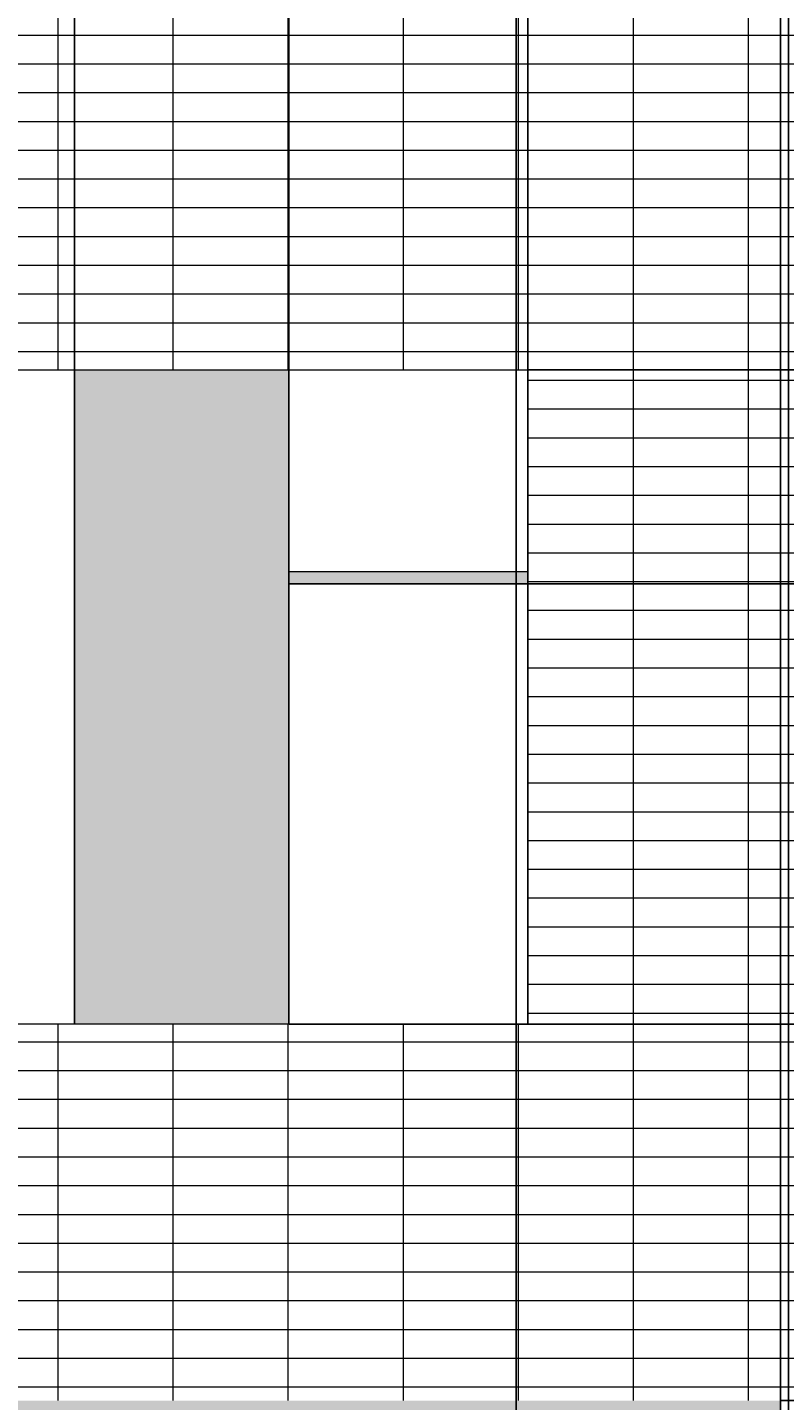
# Model space of a CAD drawing. Units: inches. Extents: x 241 to 943, y 109 to 1396.
# Tile 27 of 34: x 670 to 793, y 842 to 1065. Entities that reach past the tile are written whole.
import ezdxf

# ---------------------------------------------------------------- set-up
doc = ezdxf.new("R2010")
doc.units = ezdxf.units.IN
doc.header["$MEASUREMENT"] = 0
for name, color, linetype, lineweight in [('A-ANNO-DIMS', 2, 'Continuous', 18), ('A-ELEV-SHAD', 9, 'Continuous', 13), ('A-GLAZ', 4, 'Continuous', 18), ('A-GLAZ-PATT', 18, 'Continuous', 13), ('A-WALL-PATT', 8, 'Continuous', 13)]:
    doc.layers.add(name, color=color, linetype=linetype, lineweight=lineweight)
doc.styles.get("Standard").update_dxf_attribs({"font": 'arial.ttf'})
doc.dimstyles.get("Standard").update_dxf_attribs({"dimtxt": 1.4375, "dimasz": 0.18, "dimexe": 0.18, "dimexo": 0.0625, "dimgap": 0.09, "dimtad": 0, "dimtih": 1, "dimtoh": 1, "dimdec": 4, "dimzin": 0, "dimdsep": 46, "dimlunit": 4, "dimtxsty": 'Standard', "dimcen": 0.09, "dimadec": 0, "dimazin": 0, "dimtfac": 1, "dimtdec": 4, "dimtofl": 0, "dimtmove": 0, "dimatfit": 3, "dimfxl": 1, "dimtolj": 1, "dimtzin": 0, "dimarcsym": 0})

# ---------------------------------------------------------------- blocks, each defined once
blk = doc.blocks.new('*D14')
at = {"layer": 'A-ANNO-DIMS', "color": 0, "lineweight": -2, "transparency": 16777216}
for p, q in [((667.39, 290.06), (667.39, 1395.05)), ((667.57, 1394.87), (727.7, 1394.87)), ((793.85, 1394.87), (733.72, 1394.87)), ((794.03, 290.06), (794.03, 1395.05))]:
    blk.add_line(p, q, dxfattribs=at)
at = {"layer": 'A-ANNO-DIMS', "color": 0, "transparency": 16777216}
for points in [[(667.57, 1394.9), (667.57, 1394.84), (667.39, 1394.87)], [(793.85, 1394.9), (793.85, 1394.84), (794.03, 1394.87)]]:
    blk.add_solid(points, dxfattribs=at)
at = {"layer": 'Defpoints', "color": 0, "transparency": 16777216}
for p in [(794.03, 1394.87), (667.39, 290), (794.03, 290)]:
    blk.add_point(p, dxfattribs=at)
at = {"layer": 'A-ANNO-DIMS', "color": 0, "transparency": 16777216, "insert": (730.71, 1394.87), "char_height": 1.438, "attachment_point": 5}
blk.add_mtext('\\A1;126.63', dxfattribs=at)
blk = doc.blocks.new('*D47')
at = {"layer": 'A-ANNO-DIMS', "color": 0, "lineweight": -2, "transparency": 16777216}
for p, q in [((792.75, 841.54), (940.6, 841.54)), ((940.42, 841.36), (940.42, 789.02)), ((940.42, 735.03), (940.42, 787.37)), ((792.75, 734.85), (940.6, 734.85))]:
    blk.add_line(p, q, dxfattribs=at)
at = {"layer": 'A-ANNO-DIMS', "color": 0, "transparency": 16777216}
for points in [[(940.39, 841.36), (940.45, 841.36), (940.42, 841.54)], [(940.39, 735.03), (940.45, 735.03), (940.42, 734.85)]]:
    blk.add_solid(points, dxfattribs=at)
at = {"layer": 'Defpoints', "color": 0, "transparency": 16777216}
for p in [(792.69, 841.54), (940.42, 841.54), (792.69, 734.85)]:
    blk.add_point(p, dxfattribs=at)
at = {"layer": 'A-ANNO-DIMS', "color": 0, "transparency": 16777216, "insert": (940.42, 788.2), "char_height": 1.438, "attachment_point": 5}
blk.add_mtext('\\A1;106.68', dxfattribs=at)
blk = doc.blocks.new('*D48')
at = {"layer": 'A-ANNO-DIMS', "color": 0, "lineweight": -2, "transparency": 16777216}
for p, q in [((751.57, 1009.54), (940.6, 1009.54)), ((940.42, 1009.36), (940.42, 957.02)), ((940.42, 903.03), (940.42, 955.37)), ((751.57, 902.85), (940.6, 902.85))]:
    blk.add_line(p, q, dxfattribs=at)
at = {"layer": 'A-ANNO-DIMS', "color": 0, "transparency": 16777216}
for points in [[(940.39, 1009.36), (940.45, 1009.36), (940.42, 1009.54)], [(940.39, 903.03), (940.45, 903.03), (940.42, 902.85)]]:
    blk.add_solid(points, dxfattribs=at)
at = {"layer": 'Defpoints', "color": 0, "transparency": 16777216}
for p in [(751.51, 1009.54), (940.42, 1009.54), (751.51, 902.85)]:
    blk.add_point(p, dxfattribs=at)
at = {"layer": 'A-ANNO-DIMS', "color": 0, "transparency": 16777216, "insert": (940.42, 956.2), "char_height": 1.438, "attachment_point": 5}
blk.add_mtext('\\A1;106.68', dxfattribs=at)
blk = doc.blocks.new('*D63')
at = {"layer": 'A-ANNO-DIMS', "color": 0, "lineweight": -2, "transparency": 16777216}
for p, q in [((651.6, 568.89), (651.6, 1395.05)), ((651.78, 1394.87), (719.84, 1394.87)), ((792.51, 1394.87), (724.45, 1394.87)), ((792.69, 568.89), (792.69, 1395.05))]:
    blk.add_line(p, q, dxfattribs=at)
at = {"layer": 'A-ANNO-DIMS', "color": 0, "transparency": 16777216}
for points in [[(651.78, 1394.9), (651.78, 1394.84), (651.6, 1394.87)], [(792.51, 1394.9), (792.51, 1394.84), (792.69, 1394.87)]]:
    blk.add_solid(points, dxfattribs=at)
at = {"layer": 'Defpoints', "color": 0, "transparency": 16777216}
for p in [(792.69, 1394.87), (651.6, 568.83), (792.69, 568.83)]:
    blk.add_point(p, dxfattribs=at)
at = {"layer": 'A-ANNO-DIMS', "color": 0, "transparency": 16777216, "insert": (722.14, 1394.87), "char_height": 1.438, "attachment_point": 5}
blk.add_mtext('\\A1;141.1', dxfattribs=at)
blk = doc.blocks.new('*D64')
at = {"layer": 'A-ANNO-DIMS', "color": 0, "lineweight": -2, "transparency": 16777216}
for p, q in [((792.69, 568.89), (792.69, 1395.05)), ((792.87, 1394.87), (803.68, 1394.87)), ((820.66, 1394.87), (809.85, 1394.87)), ((820.84, 568.89), (820.84, 1395.05))]:
    blk.add_line(p, q, dxfattribs=at)
at = {"layer": 'A-ANNO-DIMS', "color": 0, "transparency": 16777216}
for points in [[(792.87, 1394.9), (792.87, 1394.84), (792.69, 1394.87)], [(820.66, 1394.9), (820.66, 1394.84), (820.84, 1394.87)]]:
    blk.add_solid(points, dxfattribs=at)
at = {"layer": 'Defpoints', "color": 0, "transparency": 16777216}
for p in [(820.84, 1394.87), (792.69, 568.83), (820.84, 568.83)]:
    blk.add_point(p, dxfattribs=at)
at = {"layer": 'A-ANNO-DIMS', "color": 0, "transparency": 16777216, "insert": (806.76, 1394.87), "char_height": 1.438, "attachment_point": 5}
blk.add_mtext('\\A1;28.146', dxfattribs=at)
blk = doc.blocks.new('*D66')
at = {"layer": 'A-ANNO-DIMS', "color": 0, "lineweight": -2, "transparency": 16777216}
for p, q in [((617.76, 702.85), (617.76, 1395.05)), ((617.94, 1394.87), (680.69, 1394.87)), ((749.45, 1394.87), (686.7, 1394.87)), ((749.63, 702.85), (749.63, 1395.05))]:
    blk.add_line(p, q, dxfattribs=at)
at = {"layer": 'A-ANNO-DIMS', "color": 0, "transparency": 16777216}
for points in [[(617.94, 1394.9), (617.94, 1394.84), (617.76, 1394.87)], [(749.45, 1394.9), (749.45, 1394.84), (749.63, 1394.87)]]:
    blk.add_solid(points, dxfattribs=at)
at = {"layer": 'Defpoints', "color": 0, "transparency": 16777216}
for p in [(749.63, 1394.87), (617.76, 702.79), (749.63, 702.79)]:
    blk.add_point(p, dxfattribs=at)
at = {"layer": 'A-ANNO-DIMS', "color": 0, "transparency": 16777216, "insert": (683.7, 1394.87), "char_height": 1.438, "attachment_point": 5}
blk.add_mtext('\\A1;131.87', dxfattribs=at)
blk = doc.blocks.new('*D68')
at = {"layer": 'A-ANNO-DIMS', "color": 0, "lineweight": -2, "transparency": 16777216}
for p, q in [((617.76, 841.6), (617.76, 1395.05)), ((617.94, 1394.87), (702.22, 1394.87)), ((792.51, 1394.87), (708.23, 1394.87)), ((792.69, 841.6), (792.69, 1395.05))]:
    blk.add_line(p, q, dxfattribs=at)
at = {"layer": 'A-ANNO-DIMS', "color": 0, "transparency": 16777216}
for points in [[(617.94, 1394.9), (617.94, 1394.84), (617.76, 1394.87)], [(792.51, 1394.9), (792.51, 1394.84), (792.69, 1394.87)]]:
    blk.add_solid(points, dxfattribs=at)
at = {"layer": 'Defpoints', "color": 0, "transparency": 16777216}
for p in [(792.69, 1394.87), (617.76, 841.54), (792.69, 841.54)]:
    blk.add_point(p, dxfattribs=at)
at = {"layer": 'A-ANNO-DIMS', "color": 0, "transparency": 16777216, "insert": (705.23, 1394.87), "char_height": 1.438, "attachment_point": 5}
blk.add_mtext('\\A1;174.93', dxfattribs=at)
blk = doc.blocks.new('*D70')
at = {"layer": 'A-ANNO-DIMS', "color": 0, "lineweight": -2, "transparency": 16777216}
for p, q in [((603.87, 1009.6), (603.87, 1395.05)), ((604.05, 1394.87), (674.69, 1394.87)), ((751.33, 1394.87), (680.69, 1394.87)), ((751.51, 1009.6), (751.51, 1395.05))]:
    blk.add_line(p, q, dxfattribs=at)
at = {"layer": 'A-ANNO-DIMS', "color": 0, "transparency": 16777216}
for points in [[(604.05, 1394.9), (604.05, 1394.84), (603.87, 1394.87)], [(751.33, 1394.9), (751.33, 1394.84), (751.51, 1394.87)]]:
    blk.add_solid(points, dxfattribs=at)
at = {"layer": 'Defpoints', "color": 0, "transparency": 16777216}
for p in [(751.51, 1394.87), (603.87, 1009.54), (751.51, 1009.54)]:
    blk.add_point(p, dxfattribs=at)
at = {"layer": 'A-ANNO-DIMS', "color": 0, "transparency": 16777216, "insert": (677.69, 1394.87), "char_height": 1.438, "attachment_point": 5}
blk.add_mtext('\\A1;147.64', dxfattribs=at)
blk = doc.blocks.new('*D71')
at = {"layer": 'A-ANNO-DIMS', "color": 0, "lineweight": -2, "transparency": 16777216}
for p, q in [((751.51, 902.92), (751.51, 1395.05)), ((751.69, 1394.87), (783.65, 1394.87)), ((820.66, 1394.87), (788.69, 1394.87)), ((820.84, 902.92), (820.84, 1395.05))]:
    blk.add_line(p, q, dxfattribs=at)
at = {"layer": 'A-ANNO-DIMS', "color": 0, "transparency": 16777216}
for points in [[(751.69, 1394.9), (751.69, 1394.84), (751.51, 1394.87)], [(820.66, 1394.9), (820.66, 1394.84), (820.84, 1394.87)]]:
    blk.add_solid(points, dxfattribs=at)
at = {"layer": 'Defpoints', "color": 0, "transparency": 16777216}
for p in [(820.84, 1394.87), (751.51, 902.85), (820.84, 902.85)]:
    blk.add_point(p, dxfattribs=at)
at = {"layer": 'A-ANNO-DIMS', "color": 0, "transparency": 16777216, "insert": (786.17, 1394.87), "char_height": 1.438, "attachment_point": 5}
blk.add_mtext('\\A1;69.33', dxfattribs=at)
blk = doc.blocks.new('*D84')
at = {"layer": 'A-ANNO-DIMS', "color": 0, "lineweight": -2, "transparency": 16777216}
for p, q in [((749.63, 702.85), (749.63, 1395.05)), ((749.81, 1394.87), (782.73, 1394.87)), ((820.66, 1394.87), (787.74, 1394.87)), ((820.84, 736.89), (820.84, 1395.05))]:
    blk.add_line(p, q, dxfattribs=at)
at = {"layer": 'A-ANNO-DIMS', "color": 0, "transparency": 16777216}
for points in [[(749.81, 1394.9), (749.81, 1394.84), (749.63, 1394.87)], [(820.66, 1394.9), (820.66, 1394.84), (820.84, 1394.87)]]:
    blk.add_solid(points, dxfattribs=at)
at = {"layer": 'Defpoints', "color": 0, "transparency": 16777216}
for p in [(820.84, 1394.87), (820.84, 736.83), (749.63, 702.79)]:
    blk.add_point(p, dxfattribs=at)
at = {"layer": 'A-ANNO-DIMS', "color": 0, "transparency": 16777216, "insert": (785.24, 1394.87), "char_height": 1.438, "attachment_point": 5}
blk.add_mtext('\\A1;71.20', dxfattribs=at)
blk = doc.blocks.new('*D87')
at = {"layer": 'A-ANNO-DIMS', "color": 0, "lineweight": -2, "transparency": 16777216}
for p, q in [((751.57, 902.85), (940.6, 902.85)), ((940.42, 902.67), (940.42, 873.02)), ((940.42, 841.72), (940.42, 871.37)), ((792.75, 841.54), (940.6, 841.54))]:
    blk.add_line(p, q, dxfattribs=at)
at = {"layer": 'A-ANNO-DIMS', "color": 0, "transparency": 16777216}
for points in [[(940.39, 902.67), (940.45, 902.67), (940.42, 902.85)], [(940.39, 841.72), (940.45, 841.72), (940.42, 841.54)]]:
    blk.add_solid(points, dxfattribs=at)
at = {"layer": 'Defpoints', "color": 0, "transparency": 16777216}
for p in [(751.51, 902.85), (940.42, 902.85), (792.69, 841.54)]:
    blk.add_point(p, dxfattribs=at)
at = {"layer": 'A-ANNO-DIMS', "color": 0, "transparency": 16777216, "insert": (940.42, 872.2), "char_height": 1.438, "attachment_point": 5}
blk.add_mtext('\\A1;61.32', dxfattribs=at)
blk = doc.blocks.new('*D88')
at = {"layer": 'A-ANNO-DIMS', "color": 0, "lineweight": -2, "transparency": 16777216}
for p, q in [((724.88, 1108.17), (940.6, 1108.17)), ((940.42, 1107.99), (940.42, 1059.68)), ((940.42, 1009.72), (940.42, 1058.03)), ((751.57, 1009.54), (940.6, 1009.54))]:
    blk.add_line(p, q, dxfattribs=at)
at = {"layer": 'A-ANNO-DIMS', "color": 0, "transparency": 16777216}
for points in [[(940.39, 1107.99), (940.45, 1107.99), (940.42, 1108.17)], [(940.39, 1009.72), (940.45, 1009.72), (940.42, 1009.54)]]:
    blk.add_solid(points, dxfattribs=at)
at = {"layer": 'Defpoints', "color": 0, "transparency": 16777216}
for p in [(724.82, 1108.17), (940.42, 1108.17), (751.51, 1009.54)]:
    blk.add_point(p, dxfattribs=at)
at = {"layer": 'A-ANNO-DIMS', "color": 0, "transparency": 16777216, "insert": (940.42, 1058.85), "char_height": 1.438, "attachment_point": 5}
blk.add_mtext('\\A1;98.63', dxfattribs=at)
blk = doc.blocks.new('*D115')
at = {"layer": 'A-ANNO-DIMS', "color": 0, "lineweight": -2, "transparency": 16777216}
for p, q in [((657.29, 902.92), (657.29, 1395.05)), ((657.47, 1394.87), (664.4, 1394.87)), ((677.51, 1394.87), (670.58, 1394.87)), ((677.69, 902.92), (677.69, 1395.05))]:
    blk.add_line(p, q, dxfattribs=at)
at = {"layer": 'A-ANNO-DIMS', "color": 0, "transparency": 16777216}
for points in [[(657.47, 1394.9), (657.47, 1394.84), (657.29, 1394.87)], [(677.51, 1394.9), (677.51, 1394.84), (677.69, 1394.87)]]:
    blk.add_solid(points, dxfattribs=at)
at = {"layer": 'Defpoints', "color": 0, "transparency": 16777216}
for p in [(677.69, 1394.87), (657.29, 902.85), (677.69, 902.85)]:
    blk.add_point(p, dxfattribs=at)
at = {"layer": 'A-ANNO-DIMS', "color": 0, "transparency": 16777216, "insert": (667.49, 1394.87), "char_height": 1.438, "attachment_point": 5}
blk.add_mtext('\\A1;20.396', dxfattribs=at)
blk = doc.blocks.new('*D116')
at = {"layer": 'A-ANNO-DIMS', "color": 0, "lineweight": -2, "transparency": 16777216}
for p, q in [((677.69, 902.92), (677.69, 1395.05)), ((677.87, 1394.87), (692.06, 1394.87)), ((712.4, 1394.87), (698.22, 1394.87)), ((712.58, 902.92), (712.58, 1395.05))]:
    blk.add_line(p, q, dxfattribs=at)
at = {"layer": 'A-ANNO-DIMS', "color": 0, "transparency": 16777216}
for points in [[(677.87, 1394.9), (677.87, 1394.84), (677.69, 1394.87)], [(712.4, 1394.9), (712.4, 1394.84), (712.58, 1394.87)]]:
    blk.add_solid(points, dxfattribs=at)
at = {"layer": 'Defpoints', "color": 0, "transparency": 16777216}
for p in [(712.58, 1394.87), (677.69, 902.85), (712.58, 902.85)]:
    blk.add_point(p, dxfattribs=at)
at = {"layer": 'A-ANNO-DIMS', "color": 0, "transparency": 16777216, "insert": (695.14, 1394.87), "char_height": 1.438, "attachment_point": 5}
blk.add_mtext('\\A1;34.895', dxfattribs=at)
blk = doc.blocks.new('*D117')
at = {"layer": 'A-ANNO-DIMS', "color": 0, "lineweight": -2, "transparency": 16777216}
for p, q in [((712.58, 902.92), (712.58, 1395.05)), ((712.76, 1394.87), (729.54, 1394.87)), ((751.33, 1394.87), (734.55, 1394.87)), ((751.51, 902.92), (751.51, 1395.05))]:
    blk.add_line(p, q, dxfattribs=at)
at = {"layer": 'A-ANNO-DIMS', "color": 0, "transparency": 16777216}
for points in [[(712.76, 1394.9), (712.76, 1394.84), (712.58, 1394.87)], [(751.33, 1394.9), (751.33, 1394.84), (751.51, 1394.87)]]:
    blk.add_solid(points, dxfattribs=at)
at = {"layer": 'Defpoints', "color": 0, "transparency": 16777216}
for p in [(751.51, 1394.87), (712.58, 902.85), (751.51, 902.85)]:
    blk.add_point(p, dxfattribs=at)
at = {"layer": 'A-ANNO-DIMS', "color": 0, "transparency": 16777216, "insert": (732.05, 1394.87), "char_height": 1.438, "attachment_point": 5}
blk.add_mtext('\\A1;38.92', dxfattribs=at)
blk = doc.blocks.new('*D118')
at = {"layer": 'A-ANNO-DIMS', "color": 0, "lineweight": -2, "transparency": 16777216}
for p, q in [((712.65, 974.63), (940.6, 974.63)), ((940.42, 974.45), (940.42, 939.55)), ((940.42, 903.03), (940.42, 937.93)), ((712.65, 902.85), (940.6, 902.85))]:
    blk.add_line(p, q, dxfattribs=at)
at = {"layer": 'A-ANNO-DIMS', "color": 0, "transparency": 16777216}
for points in [[(940.39, 974.45), (940.45, 974.45), (940.42, 974.63)], [(940.39, 903.03), (940.45, 903.03), (940.42, 902.85)]]:
    blk.add_solid(points, dxfattribs=at)
at = {"layer": 'Defpoints', "color": 0, "transparency": 16777216}
for p in [(712.58, 974.63), (940.42, 974.63), (712.58, 902.85)]:
    blk.add_point(p, dxfattribs=at)
at = {"layer": 'A-ANNO-DIMS', "color": 0, "transparency": 16777216, "insert": (940.42, 938.74), "char_height": 1.438, "attachment_point": 5}
blk.add_mtext('\\A1;71.77', dxfattribs=at)

msp = doc.modelspace()

# ---------------------------------------------------------------- hatches: boundary and pattern name
at = {"layer": 'A-ELEV-SHAD'}
h = msp.add_hatch(color=256, dxfattribs=at)
h.dxf.hatch_style = 1
h.paths.add_polyline_path([(537.4269, 698.7912), (534.1778, 698.7912), (534.1778, 659.3434), (537.4269, 659.3434)])
h.paths.add_polyline_path([(508.0803, 698.7912), (450.9259, 698.7912), (450.9259, 659.3434), (452.9259, 659.3434), (452.9259, 696.7912), (506.0803, 696.7912), (506.0803, 659.3434), (508.0803, 659.3434)])
h.paths.add_polyline_path([(481.5031, 696.7912), (479.5031, 696.7912), (479.5031, 659.3434), (481.5031, 659.3434)], flags=17)
h.paths.add_polyline_path([(481.5031, 657.3434), (479.5031, 657.3434), (479.5031, 653.3371), (481.5031, 653.3371)], flags=17)
h.paths.add_polyline_path([(508.0803, 657.3434), (506.0803, 657.3434), (506.0803, 653.3371), (452.9259, 653.3371), (452.9259, 657.3434), (450.9259, 657.3434), (450.9259, 651.3371), (508.0803, 651.3371)])
h.paths.add_polyline_path([(428.1173, 839.5382), (426.1173, 839.5382), (426.1173, 786.9154), (428.1173, 786.9154)], flags=17)
h.paths.add_polyline_path([(470.8692, 839.5382), (468.8692, 839.5382), (468.8692, 786.9154), (470.8692, 786.9154)], flags=17)
h.paths.add_polyline_path([(508.3064, 841.5382), (396.3125, 841.5382), (396.3125, 782.5808), (398.3125, 782.5808), (398.3125, 839.5382), (506.3064, 839.5382), (506.3064, 782.5808), (508.3064, 782.5808)])
h.paths.add_polyline_path([(398.3125, 780.5808), (396.3125, 780.5808), (396.3125, 773.4916), (398.3125, 773.4916)])
h.paths.add_polyline_path([(508.3064, 780.5808), (506.3064, 780.5808), (506.3064, 773.4916), (508.3064, 773.4916)])
h.paths.add_polyline_path([(715.6236, 841.5382), (678.2674, 841.5382), (678.2674, 734.8538), (715.6236, 734.8538)])
h.paths.add_polyline_path([(680.2674, 839.5382), (682.4526, 839.5382), (713.6236, 839.5382), (713.6236, 736.9235), (690.2047, 736.9235), (680.2674, 736.9235)], flags=16)
h.paths.add_polyline_path([(792.691, 841.5382), (747.7579, 841.5382), (747.7579, 734.8538), (754.5373, 734.8538), (754.5373, 736.9235), (754.5373, 839.5382), (756.7224, 839.5382), (787.8934, 839.5382), (787.8934, 765.9585), (792.691, 765.9585)])
h.paths.add_polyline_path([(659.2925, 1009.5382), (657.2925, 1009.5382), (657.2925, 902.8538), (659.2925, 902.8538)])
h.paths.add_polyline_path([(751.5078, 976.6275), (712.5839, 976.6275), (712.5839, 974.6275), (751.5078, 974.6275)])
h.paths.add_polyline_path([(470.8692, 1007.5382), (468.8692, 1007.5382), (468.8692, 954.9154), (470.8692, 954.9154)], flags=17)
h.paths.add_polyline_path([(508.3064, 1009.5382), (396.3125, 1009.5382), (396.3125, 950.5808), (398.3125, 950.5808), (398.3125, 1007.5382), (506.3064, 1007.5382), (506.3064, 950.5808), (508.3064, 950.5808)])
h.paths.add_polyline_path([(428.1173, 1007.5382), (426.1173, 1007.5382), (426.1173, 954.9154), (428.1173, 954.9154)], flags=17)
h.paths.add_polyline_path([(398.3125, 948.5808), (396.3125, 948.5808), (396.3125, 941.4916), (398.3125, 941.4916)])
h.paths.add_polyline_path([(508.3064, 948.5808), (506.3064, 948.5808), (506.3064, 941.4916), (508.3064, 941.4916)])
h.paths.add_polyline_path([(428.1173, 1175.5382), (426.1173, 1175.5382), (426.1173, 1122.9154), (428.1173, 1122.9154)], flags=17)
h.paths.add_polyline_path([(508.3064, 1177.5382), (396.3125, 1177.5382), (396.3125, 1118.5808), (398.3125, 1118.5808), (398.3125, 1175.5382), (506.3064, 1175.5382), (506.3064, 1118.5808), (506.8039, 1118.5808, -1), (506.8039, 1116.5808), (506.3064, 1116.5808), (506.3064, 1109.4916), (508.3064, 1109.4916)])
h.paths.add_polyline_path([(470.8692, 1175.5382), (468.8692, 1175.5382), (468.8692, 1122.9154), (470.8692, 1122.9154)], flags=17)
h.paths.add_polyline_path([(398.3125, 1116.5808), (396.3125, 1116.5808), (396.3125, 1109.4916), (398.3125, 1109.4916)], flags=17)
h.paths.add_polyline_path([(724.819, 1177.7336), (533.952, 1177.7336), (533.952, 1108.1686), (724.819, 1108.1686)])
h.paths.add_polyline_path([(535.952, 1175.7336), (722.819, 1175.7336), (722.819, 1110.1686), (535.952, 1110.1686)], flags=0)
h.paths.add_polyline_path([(622.521, 1136.0739), (643.4534, 1136.0739), (643.4534, 1134.0739), (622.521, 1134.0739)], flags=0)
h.paths.add_polyline_path([(722.819, 1175.7336), (535.952, 1175.7336), (535.952, 1110.1686), (722.819, 1110.1686)], flags=16)
h.paths.add_polyline_path([(565.947, 1151.5772), (535.952, 1151.5772), (535.952, 1149.5772), (565.947, 1149.5772)], flags=0)
at = {"layer": 'A-GLAZ-PATT'}
h = msp.add_hatch(dxfattribs=at)
h.set_pattern_fill('GOST_GLASS', color=256, scale=0.89)
h.set_pattern_definition([(45, (0, 0), (7.5519, 0), [4.45, -6.23]), (45, (1.888, 0), (7.5519, 0), [1.78, -8.9]), (45, (0, 1.888), (7.5519, 0), [1.78, -8.9])])
h.paths.add_polyline_path([(676.8698, 700.7912), (652.0129, 700.7912), (652.0129, 628.4013), (676.8698, 628.4013)])
h.paths.add_polyline_path([(650.0129, 700.7912), (617.7594, 700.7912), (617.7594, 628.4013), (650.0129, 628.4013)])
h.paths.add_polyline_path([(747.7579, 841.5382), (715.6236, 841.5382), (715.6236, 734.8538), (747.7579, 734.8538)])
h.paths.add_polyline_path([(678.2674, 841.5382), (642.9197, 841.5382), (642.9197, 734.8538), (678.2674, 734.8538)])
h.paths.add_polyline_path([(712.5839, 1009.5382), (677.6886, 1009.5382), (677.6886, 902.8538), (712.5839, 902.8538)])
h.paths.add_polyline_path([(640.1141, 1009.5382), (603.8694, 1009.5382), (603.8694, 902.8538), (640.1141, 902.8538)])
h.paths.add_polyline_path([(682.8748, 1175.7336), (643.4534, 1175.7336), (643.4534, 1110.1686), (682.8748, 1110.1686)])
h.paths.add_polyline_path([(602.3616, 1175.7336), (565.947, 1175.7336), (565.947, 1110.1686), (602.3616, 1110.1686)])
h = msp.add_hatch(dxfattribs=at)
h.set_pattern_fill('ANSI31', color=256, scale=34, angle=45)
h.paths.add_polyline_path([(486.3418, 786.9154), (413.1187, 786.9154), (413.1187, 761.2284), (486.3418, 761.2284)])
h.paths.add_polyline_path([(486.3418, 954.9154), (413.1187, 954.9154), (413.1187, 929.2284), (486.3418, 929.2284)])
h.paths.add_polyline_path([(462.1074, 289.6933), (390.895, 289.6933), (390.895, 277.4626), (390.895, 274.3507), (462.1074, 274.3507), (462.1074, 277.4626)])
h.paths.add_polyline_path([(500.3323, 289.6933), (479.596, 289.6933), (479.596, 274.3507), (500.3323, 274.3507)])
h.paths.add_polyline_path([(450.9259, 566.8295), (426.1086, 566.8295), (426.1086, 498.4395), (446.4348, 498.4395), (446.4348, 519.3754), (450.9259, 519.3754), (450.9259, 525.3816), (445.5808, 525.3816, -1), (445.5808, 527.3816), (450.9259, 527.3816)])
h.paths.add_polyline_path([(563.2023, 508.9074), (534.1778, 508.9074), (508.1906, 508.9074), (508.1906, 498.4395), (563.2023, 498.4395)])
h.paths.add_polyline_path([(747.6328, 700.7912), (712.0171, 700.7912), (712.0171, 628.4013), (747.6328, 628.4013)])
h.paths.add_polyline_path([(446.4348, 643.7483), (426.1086, 643.7483), (426.1086, 630.4013), (446.4348, 630.4013)])
h.paths.add_polyline_path([(564.8076, 841.5382), (553.5166, 841.5382), (508.3064, 841.5382), (508.3064, 782.5808), (564.8076, 782.5808)])
h.paths.add_polyline_path([(564.8076, 780.5808), (508.3064, 780.5808), (508.3064, 773.4916), (564.8076, 773.4916)])
h.paths.add_polyline_path([(792.691, 762.5799), (759.6248, 762.5799), (759.6248, 736.9235), (759.6248, 734.8538), (792.691, 734.8538)])
h.paths.add_polyline_path([(564.8076, 1009.5382), (553.5166, 1009.5382), (508.3064, 1009.5382), (508.3064, 950.5808), (562.3033, 950.5808, -1), (562.3033, 948.5808), (508.3064, 948.5808), (508.3064, 941.4916), (564.8076, 941.4916)])
h.paths.add_polyline_path([(486.3418, 1122.9154), (413.1187, 1122.9154), (413.1187, 1097.2284), (486.3418, 1097.2284)])
at = {"layer": 'A-WALL-PATT'}
h = msp.add_hatch(dxfattribs=at)
h.set_pattern_fill('GRATE', color=256, scale=150)
h.paths.add_polyline_path([(747.7579, 1238.8538), (747.7579, 1275.9142), (747.7579, 1336.1154), (508.3064, 1336.1154), (508.3064, 1275.9142), (508.3064, 1238.8538), (508.3064, 1177.5382), (508.3064, 1109.4916), (508.3064, 1070.8538), (553.5166, 1070.8538), (749.6328, 1070.8538)])
h.paths.add_polyline_path([(533.952, 1108.1686), (533.952, 1177.7336), (533.952, 1303.0286), (724.819, 1303.0286), (724.819, 1108.1686)], flags=16)
h.paths.add_polyline_path([(535.952, 1110.1686), (535.952, 1175.7336), (722.819, 1175.7336), (722.819, 1110.1686)], flags=0)
h.paths.add_polyline_path([(643.4534, 1134.0739), (622.521, 1134.0739), (622.521, 1136.0739), (643.4534, 1136.0739)], flags=0)
h.paths.add_polyline_path([(617.7594, 568.8295), (617.7594, 734.8538), (377.0391, 734.8538), (377.0391, 566.8538), (377.0391, 400.8295), (417.0913, 400.8295), (618.9643, 400.8295)])
h.paths.add_polyline_path([(424.1086, 496.4395), (424.1086, 568.8295), (565.2023, 568.8295), (565.2023, 496.4395)], flags=16)
h.paths.add_polyline_path([(426.1086, 498.4395), (426.1086, 566.8295), (563.2023, 566.8295), (563.2023, 508.9074), (563.2023, 498.4395)], flags=0)
h.paths.add_polyline_path([(508.0803, 508.9074), (508.0803, 519.3754), (450.9259, 519.3754), (450.9259, 525.3816), (445.5808, 525.3816, -1), (445.5808, 527.3816), (450.9259, 527.3816), (450.9259, 566.8295), (508.0803, 566.8295), (537.4269, 566.8295), (537.4269, 508.9074)], flags=0)
h.paths.add_polyline_path([(506.0803, 521.3754), (452.9259, 521.3754), (452.9259, 564.8295), (506.0803, 564.8295)], flags=0)
h.paths.add_polyline_path([(424.1086, 628.4013), (424.1086, 700.7912), (592.9542, 700.7912), (592.9542, 628.4013)], flags=16)
h.paths.add_polyline_path([(426.1086, 630.4013), (426.1086, 698.7912), (590.8792, 698.7912), (590.8792, 630.4013)], flags=0)
h.paths.add_polyline_path([(508.1906, 651.3371), (508.0803, 651.3371), (450.9259, 651.3371), (428.0291, 651.3371), (428.0291, 698.7912), (451.9767, 698.7912), (508.0803, 698.7912), (537.4269, 698.7912), (563.2023, 698.7912), (563.2023, 659.3434), (563.9297, 659.3434), (563.9297, 651.3371)], flags=0)
h.paths.add_polyline_path([(506.0803, 653.3371), (452.9259, 653.3371), (452.9259, 657.3434), (445.5808, 657.3434, -1), (445.5808, 659.3434), (452.9259, 659.3434), (452.9259, 696.7912), (506.0803, 696.7912)], flags=0)
h = msp.add_hatch(dxfattribs=at)
h.set_pattern_fill('GRATE', color=256, scale=150)
h.paths.add_polyline_path([(820.8374, 1070.8538), (749.6328, 1070.8538), (553.5166, 1070.8538), (508.3064, 1070.8538), (508.3064, 1009.5382), (553.5166, 1009.5382), (564.8076, 1009.5382), (603.8694, 1009.5382), (751.5078, 1009.5382), (751.5078, 902.8538), (603.8694, 902.8538), (603.8694, 1009.5382), (564.8076, 1009.5382), (564.8076, 941.4916), (568.1348, 941.4916), (568.1348, 902.8538), (581.3632, 902.8538), (581.3632, 841.5382), (564.8076, 841.5382), (564.8076, 782.5808), (605.9087, 782.5808, -1), (605.9087, 780.5808), (564.8076, 780.5808), (564.8076, 773.4916), (597.514, 773.4916), (607.8162, 773.4916), (607.8162, 734.8538), (617.7594, 734.8538), (617.7594, 841.5382), (792.691, 841.5382), (792.691, 734.8538), (617.7594, 734.8538), (617.7594, 702.7912), (749.6328, 702.7912), (749.6328, 626.4013), (617.7594, 626.4013), (617.7594, 568.8295), (820.8374, 568.8295), (820.8374, 736.8295), (820.8374, 902.8538)])

# ---------------------------------------------------------------- linework, layer by layer
at = {"layer": 'A-GLAZ'}
for p, q in [((677.6886, 1009.5382), (677.6886, 902.8538)), ((712.5839, 1009.5382), (712.5839, 902.8538)), ((712.5839, 976.6275), (751.5078, 976.6275)), ((712.5839, 974.6275), (751.5078, 974.6275))]:
    msp.add_line(p, q, dxfattribs=at)
msp.add_lwpolyline([(603.8694, 1009.5382), (751.5078, 1009.5382), (751.5078, 902.8538), (603.8694, 902.8538)], close=True, dxfattribs=at)

# ---------------------------------------------------------------- dimensions: what is measured, and where the dimension line sits
at = {"layer": 'A-ANNO-DIMS'}
for base, p1, p2, override, picture, middle in [((751.5078, 1394.8654), (603.8694, 1009.5382), (751.5078, 1009.5382), {"dimdec": 2, "dimlfac": 1, "dimrnd": 0, "dimzin": 0, "dimdsep": 46, "dimlunit": 2}, '*D70', (677.6886, 1394.8654)), ((749.6328, 1394.8654), (617.7594, 702.7912), (749.6328, 702.7912), {"dimdec": 2, "dimlfac": 1, "dimrnd": 0, "dimzin": 0, "dimdsep": 46, "dimlunit": 2}, '*D66', (683.6961, 1394.8654)), ((792.691, 1394.8654), (617.7594, 841.5382), (792.691, 841.5382), {"dimdec": 2, "dimlfac": 1, "dimrnd": 0, "dimzin": 0, "dimdsep": 46, "dimlunit": 2}, '*D68', (705.2252, 1394.8654)), ((792.691, 1394.8654), (651.5974, 568.8295), (792.691, 568.8295), {"dimdec": 1, "dimlfac": 1, "dimrnd": 0, "dimzin": 0, "dimdsep": 46, "dimlunit": 2}, '*D63', (722.1442, 1394.8654)), ((677.6886, 1394.8654), (657.2925, 902.8538), (677.6886, 902.8538), {"dimdec": 3, "dimlfac": 1, "dimrnd": 0, "dimzin": 0, "dimdsep": 46, "dimlunit": 2}, '*D115', (667.4905, 1394.8654)), ((794.0275, 1394.8654), (667.3935, 289.9984), (794.0275, 289.9984), {"dimdec": 2, "dimlfac": 1, "dimrnd": 0, "dimzin": 0, "dimdsep": 46, "dimlunit": 2}, '*D14', (730.7105, 1394.8654)), ((712.5839, 1394.8654), (677.6886, 902.8538), (712.5839, 902.8538), {"dimdec": 3, "dimlfac": 1, "dimrnd": 0, "dimzin": 0, "dimdsep": 46, "dimlunit": 2}, '*D116', (695.1363, 1394.8654)), ((751.5078, 1394.8654), (712.5839, 902.8538), (751.5078, 902.8538), {"dimdec": 2, "dimlfac": 1, "dimrnd": 0, "dimzin": 0, "dimdsep": 46, "dimlunit": 2}, '*D117', (732.0459, 1394.8654)), ((820.8374, 1394.8654), (749.6328, 702.7912), (820.8374, 736.8295), {"dimdec": 2, "dimlfac": 1, "dimrnd": 0, "dimzin": 0, "dimdsep": 46, "dimlunit": 2}, '*D84', (785.2351, 1394.8654)), ((820.8374, 1394.8654), (751.5078, 902.8538), (820.8374, 902.8538), {"dimdec": 2, "dimlfac": 1, "dimrnd": 0, "dimzin": 0, "dimdsep": 46, "dimlunit": 2}, '*D71', (786.1726, 1394.8654)), ((820.8374, 1394.8654), (792.691, 568.8295), (820.8374, 568.8295), {"dimdec": 3, "dimlfac": 1, "dimrnd": 0, "dimzin": 0, "dimdsep": 46, "dimlunit": 2}, '*D64', (806.7642, 1394.8654))]:
    dim = msp.add_linear_dim(base=base, p1=p1, p2=p2, dimstyle='Standard', override=override, dxfattribs=at)
    dim.commit()
    dim.dimension.update_dxf_attribs({"geometry": picture, "text_midpoint": middle})
for base, p1, p2, picture, middle in [((940.417, 1108.1686), (751.5078, 1009.5382), (724.819, 1108.1686), '*D88', (940.417, 1058.8534)), ((940.417, 1009.5382), (751.5078, 902.8538), (751.5078, 1009.5382), '*D48', (940.417, 956.196)), ((940.417, 974.6275), (712.5839, 902.8538), (712.5839, 974.6275), '*D118', (940.417, 938.7406)), ((940.417, 902.8538), (792.691, 841.5382), (751.5078, 902.8538), '*D87', (940.417, 872.196)), ((940.417, 841.5382), (792.691, 734.8538), (792.691, 841.5382), '*D47', (940.417, 788.196))]:
    dim = msp.add_linear_dim(base=base, p1=p1, p2=p2, angle=90, dimstyle='Standard', override={"dimdec": 2, "dimlfac": 1, "dimrnd": 0, "dimzin": 0, "dimdsep": 46, "dimlunit": 2}, dxfattribs=at)
    dim.commit()
    dim.dimension.update_dxf_attribs({"geometry": picture, "text_midpoint": middle})

doc.saveas('drawing.dxf')
